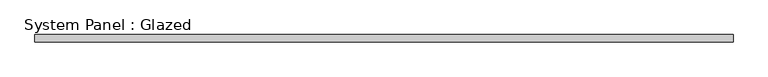
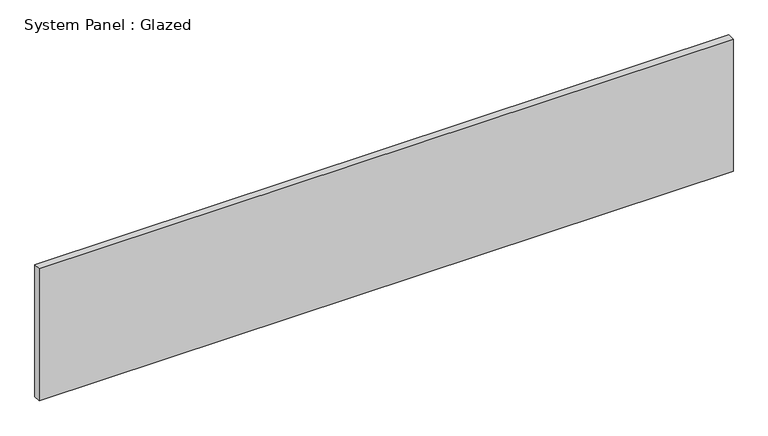
"""IFC4 building model written with IfcOpenShell, lengths in millimetres: plate geometry, System Panel : Glazed."""

from ifc_helpers import new_model, si_unit, origin, origin_with_axes, place, context, project, spatial, polyline, outline, extrude, source, transform, mapped, element, save


def system_panel_glazed_618c1181(model_context):
    return source(origin(), model_context, "Body", "SweptSolid", [
        extrude(outline(polyline([(1216.025, 19.05), (-1216.025, 19.05), (-1216.025, 44.45), (1216.025, 44.45), (1216.025, 19.05)])), origin_with_axes(), (0.0, 0.0, 1.0), 488.9673759),
    ])


if __name__ == "__main__":
    model = new_model("IFC4")
    model_context = context("Model", 3, world=origin())
    ifc_project = project(units=[si_unit("LENGTHUNIT", "METRE", prefix="MILLI")], contexts=[model_context])
    site = spatial("IfcSite", under=ifc_project)
    building = spatial("IfcBuilding", under=site)
    placement = place(None, origin())
    system_panel_glazed_shape = system_panel_glazed_618c1181(model_context)
    element("IfcPlate", 1, ObjectType="System Panel : Glazed", at=placement, inside=building, context=model_context, shape_type="MappedRepresentation", body=[
        mapped(system_panel_glazed_shape, transform((0.0, 0.0, 0.0), x_axis=(1.0, 0.0, 0.0), y_axis=(0.0, 1.0, 0.0), z_axis=(0.0, 0.0, 1.0))),
    ])
    save(model, "model.ifc")

# Revit data of these elements
# Type "System Panel : Glazed"
#   Construction Type Id = "GSP4R"
#   Analytic Construction = "1/8 in Pilkington single glazing"
#   Visual Light Transmittance = 0.9
#   Solar Heat Gain Coefficient = 0.86
#   Heat Transfer Coefficient (U) = 1.18115 BTU/(h·ft²·°F)
#   Define Thermal Properties by = 1
# Element 1 (IfcPlate, "System Panel : Glazed")
#   Materials on its faces: "Glass"
# Materials
#   "Glass": class "Glass", colour RGB 0 128 192, transparency 0.75, Description = "Soda Lime Glass", Cost = 0
